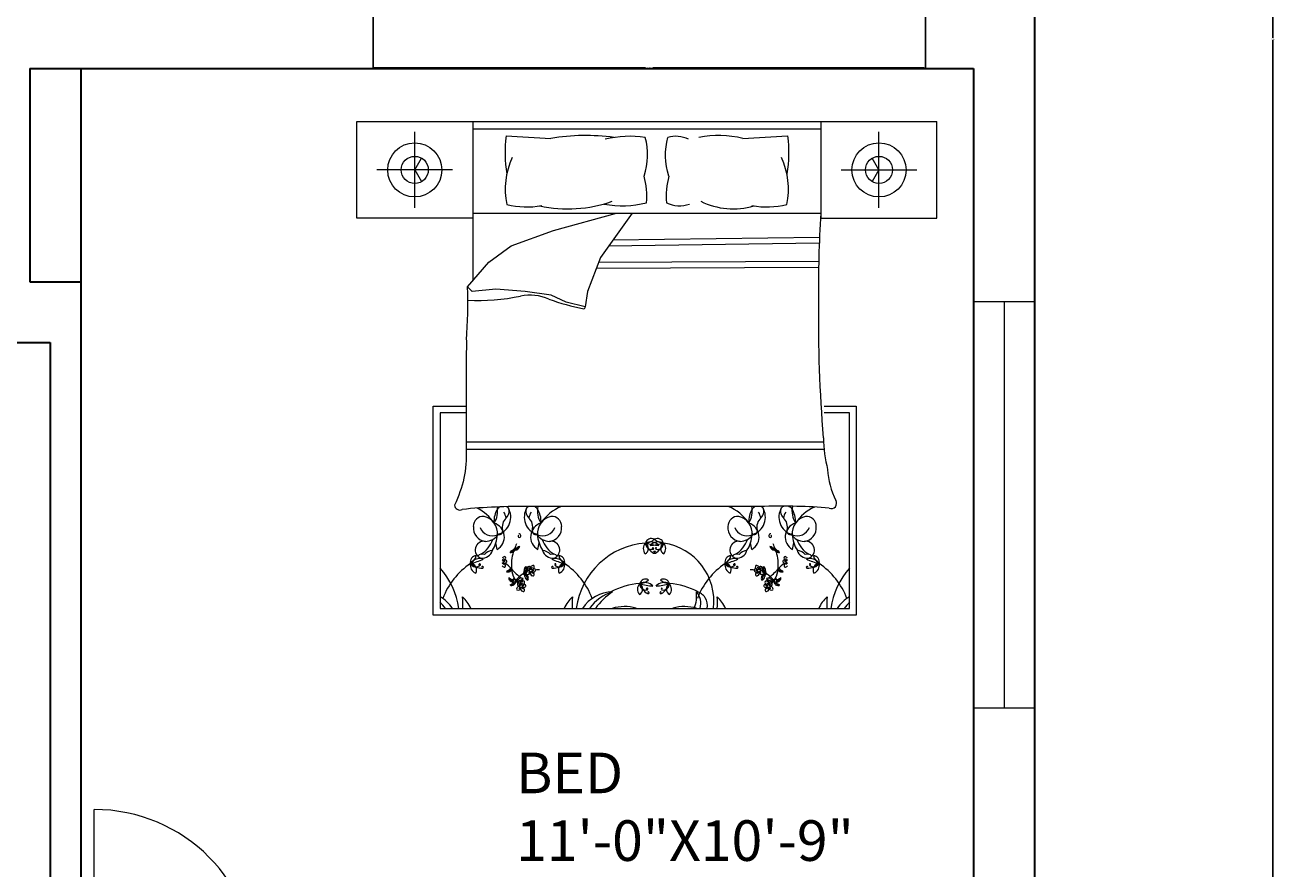
# Model space of a CAD drawing. Units: inches. Extents: x -59 to 444, y -680 to 63.
# Tile 7 of 9: x 260 to 444, y -431 to -306. Entities that reach past the tile are written whole.
import ezdxf

# ---------------------------------------------------------------- set-up
doc = ezdxf.new("R2010")
doc.units = ezdxf.units.IN
doc.header["$MEASUREMENT"] = 0
for name, color, linetype, lineweight in [('A-ANNO-DIMS', 2, 'Continuous', 18), ('A-AREA-IDEN', 7, 'Continuous', 18), ('A-DOOR', 3, 'Continuous', 18), ('A-FLOR-EVTR', 7, 'Continuous', 30), ('A-FURN', 8, 'Continuous', 13), ('A-GLAZ', 4, 'Continuous', 18), ('A-WALL', 7, 'Continuous', 35)]:
    doc.layers.add(name, color=color, linetype=linetype, lineweight=lineweight)
doc.styles.get("Standard").update_dxf_attribs({"font": 'arial.ttf'})
doc.dimstyles.get("Standard").update_dxf_attribs({"dimtxt": 0.18, "dimasz": 0.18, "dimexe": 0.18, "dimexo": 0.0625, "dimgap": 0.09, "dimtad": 0, "dimtih": 1, "dimtoh": 1, "dimdec": 0, "dimzin": 0, "dimdsep": 46, "dimlunit": 3, "dimtxsty": 'Standard', "dimcen": 0.09, "dimadec": 0, "dimazin": 0, "dimtfac": 1, "dimtdec": 0, "dimtofl": 0, "dimtmove": 0, "dimatfit": 3, "dimfxl": 1, "dimtolj": 1, "dimtzin": 0, "dimarcsym": 0})

# ---------------------------------------------------------------- blocks, each defined once
blk = doc.blocks.new('BED-SET-73')
for p, q in [((0, 72.95), (85.77, 72.95)), ((17.15, 72.95), (17.15, 49.4)), ((8.58, 60.19), (8.58, 71.4)), ((68.62, 71.84), (17.15, 71.84)), ((77.2, 60.19), (77.2, 71.4)), ((14.18, 65.8), (2.97, 65.8)), ((71.59, 65.8), (82.8, 65.8)), ((17.15, 59.39), (68.62, 59.39)), ((29.07, 56.84), (38.42, 59.39)), ((40.72, 59.39), (36.02, 52.85)), ((22.81, 54.58), (29.07, 56.84)), ((68.39, 55.83), (37.85, 55.4)), ((19.51, 52.15), (22.81, 54.58)), ((68.36, 54.95), (37.21, 54.51)), ((16.39, 48.51), (19.51, 52.15)), ((36.02, 52.85), (34.11, 47.81)), ((68.31, 52.25), (35.74, 52.12)), ((68.32, 51.37), (35.4, 51.23)), ((17.08, 47.81), (16.39, 48.51)), ((20.56, 48.16), (17.08, 47.81)), ((24.9, 47.81), (20.56, 48.16)), ((28.72, 47.29), (24.9, 47.81)), ((30.98, 46.25), (28.72, 47.29)), ((33.76, 45.56), (30.98, 46.25)), ((34.11, 47.81), (33.76, 45.56)), ((11.32, 30.9), (16.17, 30.9)), ((11.32, 0), (11.32, 30.9)), ((16.17, 29.9), (12.32, 29.9)), ((12.32, 29.9), (12.32, 0.99)), ((72.86, 29.9), (69.08, 29.9)), ((69.1, 30.9), (73.85, 30.9)), ((72.86, 0.99), (72.86, 29.9)), ((73.85, 30.9), (73.85, 0)), ((69.01, 25.55), (16.17, 25.55)), ((69.09, 24.48), (16.17, 24.48)), ((60.3, 16.05), (25.47, 16.05)), ((20.77, 9.69), (20.58, 10.66)), ((26.76, 9.69), (26.95, 10.66)), ((58.41, 9.69), (58.22, 10.66)), ((64.41, 9.69), (64.6, 10.66)), ((73.85, 0), (11.32, 0)), ((12.32, 0.99), (72.86, 0.99))]:
    blk.add_line(p, q)
for points in [[(17.15, 58.65), (0, 58.65), (0, 72.95)], [(68.62, 72.95), (68.62, 58.65), (85.77, 58.65), (85.77, 72.95)], [(8.58, 65.8), (9.58, 67.53)], [(77.2, 65.8), (76.2, 67.53)], [(8.58, 65.8), (9.58, 64.06)], [(77.2, 65.8), (76.2, 64.06)]]:
    blk.add_lwpolyline(points)
for points in [[(22.08, 70.81, 0.074897), (22.19, 65.21, -0.472817)], [(42.49, 64.89, 0.14099), (42.66, 70.61, 0.235245)], [(46.15, 64.89, -0.14099), (45.98, 70.61, -0.235245)], [(63.69, 70.81, -0.074897), (63.59, 65.21, 0.472817)], [(16.21, 40.65, 0.001242), (16.17, 24.38, -0.127202), (14.45, 16.27)], [(68.99, 26.22, 0.056112), (69.61, 21.51, 0.095341), (70.81, 16.96)]]:
    blk.add_lwpolyline(points, format="xyb")
for centre, radius in [((8.58, 65.8), 4), ((77.2, 65.8), 4), ((8.58, 65.8), 2), ((77.2, 65.8), 2), ((25.72, 6.58), 0.218), ((59.45, 6.58), 0.218), ((24.29, 4.28), 0.218), ((60.88, 4.28), 0.218)]:
    blk.add_circle(centre, radius)
for centre, radius, start, end in [((69.36, 887.1), 817.66, 266.68521, 267.14978), ((33.83, 39.77), 31.11, 82.2196, 99.497), ((40.4, 55.49), 15.28, 81.5249, 103.96), ((47.15, 66.53), 4.24, 63.3437, 106.1026), ((53.51, 55.8), 15.08, 76.3427, 101.1841), ((16.41, 887.1), 817.66, 272.85022, 273.31479), ((33.01, 62.96), 11.06, 155.1316, 191.7583), ((52.76, 62.96), 11.06, 348.2417, 24.8684), ((32.37, 62.02), 10.51, 354.0129, 15.8293), ((56.26, 62.02), 10.51, 164.1707, 185.9871), ((31.19, 79.98), 19.94, 258.0397, 289.2615), ((55.67, 70.96), 10.92, 243.8761, 286.1746), ((25.14, 71.81), 11.49, 255.1039, 281.0369), ((39.26, 75.63), 15.13, 259.8617, 283.6238), ((47.73, 65.05), 4.55, 245.0183, 288.5407), ((60.63, 71.81), 11.49, 258.9631, 284.8961), ((222.38, 48.91), 154.12, 176.1, 180.9282), ((-62.26, 46.38), 78.68, 355.8294, 1.553), ((17.85, 78.88), 32.37, 267.4519, 281.3392), ((25.59, 40.3), 6.98, 66.2616, 101.3392), ((39.72, 77.97), 33.26, 250.1194, 259.3383), ((269.3, 43.3), 201.05, 179.1145, 184.8735), ((33.57, 45.49), 0.207, 268.8623, 19.7536), ((70.16, 16.52), 0.782, 246.5219, 33.8264), ((15.24, 16.32), 0.791, 183.98, 297.3412), ((24.45, -73.23), 89.29, 89.3433, 95.6887), ((14.9, 10.01), 6.49, 33.6671, 63.2997), ((23.6, 13.88), 3.31, 145.785, 184.7304), ((17.28, 15.42), 3.55, 328.8218, 9.1554), ((21.68, 15.1), 1.03, 120.0293, 142.325), ((20.04, 14.5), 2.73, 289.2822, 29.1751), ((19.62, 14), 2.47, 7.436, 29.9149), ((21.25, 15.31), 1.28, 311.5653, 23.8354), ((21.68, 15.1), 1.03, 44.4517, 63.558), ((27.5, 14.5), 2.73, 150.8249, 250.7178), ((26.28, 15.31), 1.28, 156.1646, 228.4347), ((25.85, 15.1), 1.03, 113.229, 135.5483), ((27.91, 14), 2.47, 150.0851, 172.564), ((25.85, 15.1), 1.03, 37.675, 66.7144), ((23.93, 13.88), 3.31, 355.2696, 34.215), ((30.25, 15.42), 3.55, 169.7133, 211.1782), ((32.63, 10.01), 6.49, 111.4941, 146.3329), ((52.55, 10.01), 6.49, 33.6671, 68.5059), ((61.25, 13.88), 3.31, 145.785, 184.7304), ((54.93, 15.42), 3.55, 328.8218, 10.2867), ((59.33, 15.1), 1.03, 113.2856, 142.325), ((57.68, 14.5), 2.73, 289.2822, 29.1751), ((57.27, 14), 2.47, 7.436, 29.9149), ((59.33, 15.1), 1.03, 44.4517, 66.7144), ((58.89, 15.31), 1.28, 311.5653, 23.8354), ((62.93, -67.37), 83.47, 85.2402, 91.8035), ((65.14, 14.5), 2.73, 150.8249, 250.7178), ((63.93, 15.31), 1.28, 156.1646, 228.4347), ((63.49, 15.1), 1.03, 106.6343, 135.5483), ((65.55, 14), 2.47, 150.0851, 172.564), ((63.49, 15.1), 1.03, 37.675, 72.5814), ((61.57, 13.88), 3.31, 355.2696, 34.215), ((67.89, 15.42), 3.55, 169.249, 211.1782), ((70.27, 10.01), 6.49, 113.6453, 146.3329), ((19.28, 12.92), 2.05, 174.9449, 262.8857), ((18.68, 13.13), 1.45, 84.4856, 181.0538), ((20.08, 13.7), 1.99, 201.5819, 291.4221), ((18.24, 12.06), 2.58, 355.2933, 76.921), ((19.7, 11.54), 2.13, 299.9085, 73.1337), ((23.27, 13.03), 1.76, 131.5653, 195.1471), ((24.26, 13.03), 1.76, 344.8529, 48.4347), ((27.83, 11.54), 2.13, 106.8663, 240.0915), ((29.29, 12.06), 2.58, 103.079, 184.7067), ((27.45, 13.7), 1.99, 248.5779, 338.4181), ((28.25, 12.92), 2.05, 277.1143, 5.0551), ((28.85, 13.13), 1.45, 358.9462, 95.5144), ((56.92, 12.92), 2.05, 174.9449, 262.8857), ((56.33, 13.13), 1.45, 84.4856, 181.0538), ((57.73, 13.7), 1.99, 201.5819, 291.4221), ((55.88, 12.06), 2.58, 355.2933, 76.921), ((57.35, 11.54), 2.13, 299.9085, 73.1337), ((60.91, 13.03), 1.76, 131.5653, 195.1471), ((61.91, 13.03), 1.76, 344.8529, 48.4347), ((65.47, 11.54), 2.13, 106.8663, 240.0915), ((66.94, 12.06), 2.58, 103.079, 184.7067), ((65.09, 13.7), 1.99, 248.5779, 338.4181), ((65.9, 12.92), 2.05, 277.1143, 5.0551), ((66.49, 13.13), 1.45, 358.9462, 95.5144), ((16.25, 12.45), 4.05, 301.2614, 341.7045), ((18.92, 13.38), 2.49, 272.3591, 324.0401), ((16.22, 12.13), 4.6, 326.2883, 356.5076), ((23.6, 13.88), 3.31, 212.7011, 216.3445), ((21.05, 12.43), 0.532, 257.3041, 15.1471), ((24.01, 11.63), 0.165, 102.7051, 280.4384), ((23.99, 11.73), 0.269, 280.4384, 100.4136), ((26.48, 12.43), 0.532, 164.8529, 282.6959), ((23.93, 13.88), 3.31, 323.6555, 327.2989), ((28.61, 13.38), 2.49, 215.9599, 267.6409), ((31.31, 12.13), 4.6, 183.4924, 213.7117), ((31.28, 12.45), 4.05, 198.2955, 238.7386), ((43.57, 10.39), 0.929, 63.0274, 163.8037), ((42.63, 12.56), 1.91, 271.4585, 315.3727), ((44.46, 10.39), 0.929, 16.1963, 116.9726), ((45.4, 12.56), 1.91, 224.6273, 268.5415), ((53.9, 12.45), 4.05, 301.2614, 341.7045), ((56.57, 13.38), 2.49, 272.3591, 324.0401), ((53.86, 12.13), 4.6, 326.2883, 356.5076), ((61.25, 13.88), 3.31, 212.7011, 216.3445), ((58.7, 12.43), 0.532, 257.3041, 15.1471), ((61.18, 11.73), 0.269, 79.5864, 259.5616), ((61.16, 11.63), 0.165, 259.5616, 77.2949), ((64.12, 12.43), 0.532, 164.8529, 282.6959), ((61.57, 13.88), 3.31, 323.6555, 327.2989), ((66.25, 13.38), 2.49, 215.9599, 267.6409), ((68.96, 12.13), 4.6, 183.4924, 213.7117), ((68.92, 12.45), 4.05, 198.2955, 238.7386), ((18.81, 9.62), 1.29, 80.264, 250.8688), ((18.5, 10.01), 1.61, 265.969, 344.3045), ((20.23, 7.87), 1.71, 96.1662, 141.5825), ((23.06, 9.07), 0.45, 101.3256, 154.4621), ((22.42, 10.6), 1.36, 280.2588, 300.656), ((22.73, 11.68), 2.42, 268.3264, 277.1302), ((29.96, 7.31), 7.1, 163.5842, 183.8277), ((22.12, 10.6), 1.38, 308.2101, 316.3071), ((22.97, 9.69), 0.412, 278.3432, 4.2869), ((22.74, 10.05), 0.719, 300.656, 332.6341), ((23.28, 9.58), 0.175, 55.7657, 157.4417), ((29.96, 7.31), 7.1, 153.0032, 159.8941), ((23.55, 9.74), 0.175, 84.3784, 186.0543), ((23.39, 10.44), 0.719, 269.1859, 301.164), ((23.6, 10.07), 0.412, 237.5332, 323.4768), ((23.2, 11.24), 1.38, 285.5129, 293.6099), ((24.1, 9.69), 0.45, 87.3579, 140.4944), ((23.06, 10.99), 1.36, 301.164, 321.5612), ((21.96, 11.22), 2.42, 324.6898, 333.4936), ((27.3, 7.87), 1.71, 38.4175, 83.8338), ((29.03, 10.01), 1.61, 195.6955, 274.031), ((28.72, 9.62), 1.29, 289.1312, 99.736), ((43.55, -0.52), 11.2, 94.4623, 172.255), ((43.6, 9.82), 1.24, 137.7873, 219.1145), ((42.19, 9.86), 0.935, 298.5391, 58.3627), ((43.41, 9.04), 1.77, 45.5411, 114.3101), ((45.03, 18.13), 7.84, 252.593, 267.2582), ((43.6, 10.62), 0.916, 177.7585, 283.852), ((45.36, 11.57), 2.83, 198.9159, 238.011), ((44.62, 9.04), 1.77, 65.6899, 134.4589), ((43.01, 18.13), 7.84, 272.7418, 287.407), ((43.79, 9.84), 0.121, 283.852, 219.9245), ((43.94, 9.29), 0.139, 238.011, 71.5592), ((43.96, 9.35), 0.0676, 71.5592, 188.0167), ((44.1, 9.29), 0.139, 108.4408, 301.989), ((44.08, 9.35), 0.0676, 351.9833, 108.4408), ((44.23, 9.89), 0.073, 320.1909, 256.0209), ((42.67, 11.57), 2.83, 301.989, 341.0841), ((44.44, 10.62), 0.916, 256.148, 2.2415), ((45.84, 9.86), 0.935, 121.6373, 241.4609), ((44.43, 9.82), 1.24, 320.8855, 42.2127), ((44.12, 2.07), 8.67, 352.8636, 81.8197), ((56.45, 9.62), 1.29, 80.264, 250.8688), ((56.14, 10.01), 1.61, 265.969, 344.3045), ((57.87, 7.87), 1.71, 96.1662, 141.5825), ((62.12, 10.99), 1.36, 218.4388, 238.836), ((61.07, 9.69), 0.45, 39.5056, 92.6421), ((63.22, 11.22), 2.42, 206.5064, 215.3102), ((61.58, 10.07), 0.412, 216.5232, 302.4668), ((61.79, 10.44), 0.719, 238.836, 270.8141), ((61.97, 11.24), 1.38, 246.3901, 254.4871), ((55.22, 7.31), 7.1, 20.1059, 26.9968), ((61.62, 9.74), 0.175, 353.9457, 95.6216), ((61.89, 9.58), 0.175, 22.5583, 124.2343), ((62.21, 9.69), 0.412, 175.7131, 261.6568), ((62.43, 10.05), 0.719, 207.3659, 239.344), ((55.22, 7.31), 7.1, 356.1723, 16.4158), ((63.05, 10.6), 1.38, 223.6929, 231.7899), ((62.76, 10.6), 1.36, 239.344, 259.7412), ((62.45, 11.68), 2.42, 262.8698, 271.6736), ((62.11, 9.07), 0.45, 25.5379, 78.6744), ((66.68, 10.01), 1.61, 195.6955, 274.031), ((64.95, 7.87), 1.71, 38.4175, 83.8338), ((66.37, 9.62), 1.29, 289.1312, 99.736), ((23.14, -1.62), 11.2, 124.3865, 158.5908), ((18.03, 7.36), 1.24, 167.7115, 249.0387), ((17.72, 7.84), 0.929, 92.9516, 193.728), ((15.82, 9.25), 1.91, 301.3827, 345.2969), ((18.25, 6.59), 1.77, 75.4653, 144.2343), ((15.12, 15.27), 7.84, 282.5173, 297.1824), ((16.79, 6.69), 0.935, 328.4633, 88.2869), ((18.68, 9.75), 2.83, 228.8402, 267.9352), ((17.62, 8.05), 0.916, 207.6827, 313.7762), ((18.54, 8.23), 0.789, 63.9755, 143.2681), ((18.17, 7.47), 0.121, 313.7762, 249.7183), ((21.79, 8.22), 0.364, 101.5637, 142.6358), ((21.49, 7.88), 0.218, 273.2768, 86.7232), ((21.74, 8.09), 0.209, 91.1081, 181.8675), ((22.18, 7.96), 0.663, 203.4276, 227.6104), ((21.96, 7.67), 0.452, 80.3487, 133.6538), ((21.88, 8.04), 0.357, 229.7889, 317.6792), ((21.5, 8.5), 0.525, 288.7263, 352.5032), ((21.48, 7.28), 0.508, 355.053, 68.3618), ((21.88, 7.2), 0.715, 83.0852, 105.7171), ((21.86, 8.48), 0.169, 345.2356, 144.9248), ((16.93, 1.27), 8.14, 43.1541, 52.0459), ((22.01, 7.93), 0.188, 317.6792, 80.3487), ((28.99, 8.23), 0.789, 36.7319, 116.0245), ((29.28, 6.59), 1.77, 35.7657, 104.5347), ((32.42, 15.27), 7.84, 242.8176, 257.4827), ((28.85, 9.75), 2.83, 272.0648, 311.1598), ((29.91, 8.05), 0.916, 226.2238, 332.3173), ((29.37, 7.52), 0.073, 290.2667, 226.2271), ((30.74, 6.69), 0.935, 91.7131, 211.5367), ((29.81, 7.84), 0.929, 346.272, 87.0484), ((31.71, 9.25), 1.91, 194.7031, 238.6173), ((29.5, 7.36), 1.24, 290.9613, 12.2885), ((24.39, -1.62), 11.2, 21.4092, 55.6135), ((60.78, -1.62), 11.2, 124.3865, 158.5908), ((55.36, 7.84), 0.929, 92.9516, 193.728), ((55.67, 7.36), 1.24, 167.7115, 249.0387), ((53.46, 9.25), 1.91, 301.3827, 345.2969), ((55.9, 6.59), 1.77, 75.4653, 144.2343), ((52.76, 15.27), 7.84, 282.5173, 297.1824), ((55.27, 8.05), 0.916, 207.6827, 313.7762), ((56.32, 9.75), 2.83, 228.8402, 267.9352), ((54.43, 6.69), 0.935, 328.4633, 88.2869), ((56.19, 8.23), 0.789, 63.9755, 143.2681), ((55.82, 7.47), 0.121, 313.7762, 249.7183), ((68.25, 1.27), 8.14, 127.9541, 136.8459), ((63.17, 7.93), 0.188, 99.6513, 222.3208), ((63.29, 8.04), 0.357, 222.3208, 310.2111), ((63.21, 7.67), 0.452, 46.3462, 99.6513), ((63.32, 8.48), 0.169, 35.0752, 194.7644), ((63.68, 8.5), 0.525, 187.4968, 251.2737), ((63.69, 7.28), 0.508, 111.6382, 184.947), ((63.3, 7.2), 0.715, 74.2829, 96.9148), ((63.43, 8.09), 0.209, 358.1325, 88.8919), ((63, 7.96), 0.663, 312.3896, 336.5724), ((63.38, 8.22), 0.364, 37.3642, 78.4363), ((63.69, 7.88), 0.218, 93.2768, 266.7232), ((66.63, 8.23), 0.789, 36.7319, 116.0245), ((66.93, 6.59), 1.77, 35.7657, 104.5347), ((70.06, 15.27), 7.84, 242.8176, 257.4827), ((66.5, 9.75), 2.83, 272.0648, 311.1598), ((67.55, 8.05), 0.916, 226.2238, 332.3173), ((67.01, 7.52), 0.073, 290.2667, 226.2271), ((68.39, 6.69), 0.935, 91.7131, 211.5367), ((69.36, 9.25), 1.91, 194.7031, 238.6173), ((67.46, 7.84), 0.929, 346.272, 87.0484), ((67.15, 7.36), 1.24, 290.9613, 12.2885), ((62.04, -1.62), 11.2, 21.4092, 55.6135), ((3.98, -0.52), 11.2, 7.745, 41.8856), ((18.57, 7.13), 0.0676, 101.4834, 217.9409), ((18.58, 7.06), 0.139, 267.9352, 101.4834), ((21.79, 7.48), 0.361, 217.7621, 259.0403), ((21.82, 7.25), 0.168, 232.4737, 355.053), ((22.55, 6.19), 0.45, 101.3256, 154.4621), ((21.91, 7.71), 1.36, 280.2588, 300.656), ((22.22, 8.8), 2.42, 268.3264, 277.1302), ((21.61, 7.71), 1.38, 308.2101, 316.3071), ((22.46, 6.81), 0.412, 278.3432, 4.2869), ((22.23, 7.17), 0.719, 300.656, 332.6341), ((22.77, 6.69), 0.175, 55.7657, 157.4417), ((26.42, 7.13), 3.56, 184.756, 209.2041), ((31.54, 14.71), 11.72, 222.2412, 232.1744), ((26.78, 2.4), 4.27, 120.544, 139.818), ((24.58, 6.68), 0.605, 272.8499, 356.1226), ((24.05, 6.91), 0.996, 304.5369, 16.3699), ((24.16, 6.45), 0.586, 321.7607, 7.9252), ((24.28, 5.61), 0.586, 8.7227, 54.8872), ((24.31, 5.14), 0.996, 0.278, 72.111), ((25.43, 6.63), 0.704, 127.3105, 187.9252), ((24.76, 5.5), 0.605, 20.5253, 88.5375), ((25.55, 5.8), 0.704, 188.7227, 249.3375), ((24.47, 6.71), 0.723, 355.0106, 41.658), ((25.26, 6.17), 0.216, 148.0499, 225.6268), ((26.78, 2.4), 4.27, 113.0501, 113.8477), ((25.66, 5.92), 0.689, 104.7558, 148.0499), ((25.28, 6.42), 0.431, 247.4086, 351.4386), ((25.48, 6.89), 0.298, 126.1046, 271.4281), ((25.45, 6.97), 0.214, 353.7526, 131.7054), ((24.65, 5.45), 0.723, 334.9899, 21.6373), ((25.4, 6.4), 0.145, 262.906, 7.132), ((25.25, 6.71), 0.301, 0.0645, 61.1507), ((25.32, 6.97), 0.344, 311.8413, 355.7877), ((26.03, 6.92), 0.364, 101.5637, 176.365), ((26.02, 6.18), 0.361, 151.2196, 259.0403), ((25.98, 6.79), 0.209, 91.1081, 181.8675), ((26.41, 6.66), 0.663, 203.4276, 227.6104), ((26.2, 6.37), 0.452, 80.3487, 133.6538), ((26.12, 6.74), 0.357, 229.7889, 317.6792), ((25.73, 7.21), 0.525, 288.7263, 352.5032), ((25.72, 5.99), 0.508, 355.053, 68.3618), ((26.11, 5.9), 0.715, 83.0852, 105.7171), ((26.09, 7.18), 0.169, 345.2356, 144.9248), ((26.05, 5.96), 0.168, 232.4737, 355.053), ((26.24, 6.63), 0.188, 317.6792, 80.3487), ((26.78, 2.4), 4.27, 87.1071, 94.7585), ((28.95, 7.06), 0.139, 78.5166, 272.0648), ((28.96, 7.13), 0.0676, 322.0591, 78.5166), ((56.21, 7.13), 0.0676, 101.4834, 217.9409), ((56.23, 7.06), 0.139, 267.9352, 101.4834), ((58.39, 2.4), 4.27, 85.2415, 92.8929), ((58.93, 6.63), 0.188, 99.6513, 222.3208), ((59.06, 6.74), 0.357, 222.3208, 310.2111), ((58.98, 6.37), 0.452, 46.3462, 99.6513), ((59.09, 7.18), 0.169, 35.0752, 194.7644), ((59.44, 7.21), 0.525, 187.4968, 251.2737), ((59.46, 5.99), 0.508, 111.6382, 184.947), ((59.12, 5.96), 0.168, 184.947, 307.5263), ((59.06, 5.9), 0.715, 74.2829, 96.9148), ((59.2, 6.79), 0.209, 358.1325, 88.8919), ((58.77, 6.66), 0.663, 312.3896, 336.5724), ((59.15, 6.92), 0.364, 3.635, 78.4363), ((59.15, 6.18), 0.361, 280.9597, 28.7804), ((59.9, 6.42), 0.431, 188.5614, 292.5914), ((59.73, 6.97), 0.214, 48.2946, 186.2474), ((59.86, 6.97), 0.344, 184.2123, 228.1587), ((59.93, 6.71), 0.301, 118.8493, 179.9355), ((59.78, 6.4), 0.145, 172.868, 277.094), ((59.69, 6.89), 0.298, 268.5719, 53.8954), ((59.51, 5.92), 0.689, 31.9501, 75.2442), ((60.53, 5.45), 0.723, 158.3627, 205.0101), ((60.42, 5.5), 0.605, 91.4625, 159.4747), ((60.87, 5.14), 0.996, 107.889, 179.722), ((59.62, 5.8), 0.704, 290.6625, 351.2773), ((60.71, 6.71), 0.723, 138.342, 184.9894), ((60.59, 6.68), 0.605, 183.8774, 267.1501), ((58.39, 2.4), 4.27, 66.1523, 66.9499), ((59.91, 6.17), 0.216, 314.3732, 31.9501), ((61.12, 6.91), 0.996, 163.6301, 235.4631), ((59.74, 6.63), 0.704, 352.0748, 52.6895), ((60.9, 5.61), 0.586, 125.1128, 171.2773), ((61.02, 6.45), 0.586, 172.0748, 218.2393), ((58.39, 2.4), 4.27, 40.182, 59.456), ((53.63, 14.71), 11.72, 307.8256, 317.7588), ((58.76, 7.13), 3.56, 330.7959, 355.244), ((62.41, 6.69), 0.175, 22.5583, 124.2343), ((62.72, 6.81), 0.412, 175.7131, 261.6568), ((62.95, 7.17), 0.719, 207.3659, 239.344), ((63.56, 7.71), 1.38, 223.6929, 231.7899), ((63.27, 7.71), 1.36, 239.344, 259.7412), ((62.96, 8.8), 2.42, 262.8698, 271.6736), ((62.62, 6.19), 0.45, 25.5379, 78.6744), ((63.36, 7.25), 0.168, 184.947, 307.5263), ((63.39, 7.48), 0.361, 280.9597, 322.2379), ((66.59, 7.06), 0.139, 78.5166, 272.0648), ((66.61, 7.13), 0.0676, 322.0591, 78.5166), ((81.2, -0.52), 11.2, 138.1144, 172.255), ((22.71, 5.4), 0.244, 146.8636, 236.9021), ((26.14, 10.77), 6.38, 235.1882, 238.8844), ((23.12, 5.75), 0.66, 199.4799, 267.6828), ((23.05, 5.5), 0.569, 212.8155, 277.3992), ((22.72, 5.12), 0.66, 266.9701, 338.2913), ((19.24, 9.83), 6.38, 302.6784, 306.3746), ((22.89, 4.6), 0.244, 214.3538, 304.3923), ((22.98, 5.52), 0.253, 238.8844, 314.2646), ((22.92, 4.96), 0.569, 280.3057, 17.1958), ((22.87, 4.9), 0.253, 306.3746, 21.7548), ((23.29, 5.06), 0.191, 19.3605, 201.7548), ((23.29, 5.2), 0.191, 311.8703, 134.2646), ((26.87, 3.47), 3.8, 153.7819, 158.2913), ((23.84, 6.07), 0.996, 247.2305, 319.0635), ((23.51, 5.73), 0.586, 264.4544, 310.6188), ((23.94, 5.5), 0.605, 218.3208, 298.8162), ((26.42, 7.13), 3.56, 214.0033, 222.4917), ((23.84, 3.87), 0.216, 148.0499, 225.6268), ((24.24, 3.62), 0.689, 104.7558, 148.0499), ((23.85, 4.11), 0.431, 247.4086, 351.4386), ((24.05, 4.58), 0.298, 126.1046, 271.4281), ((24.02, 4.66), 0.214, 353.7526, 131.7054), ((24.35, 4.75), 0.704, 70.0041, 130.6188), ((23.97, 4.1), 0.145, 262.906, 7.132), ((23.82, 4.41), 0.301, 0.0645, 61.1507), ((23.89, 4.67), 0.344, 311.8413, 355.7877), ((23.89, 5.61), 0.723, 297.7043, 344.3516), ((24.6, 4.62), 0.364, 101.5637, 176.365), ((24.59, 3.88), 0.361, 151.2196, 259.0403), ((24.55, 4.49), 0.209, 91.1081, 181.8675), ((24.98, 4.36), 0.663, 203.4276, 227.6104), ((24.77, 4.07), 0.452, 80.3487, 133.6538), ((24.69, 4.44), 0.357, 229.7889, 317.6792), ((24.3, 4.9), 0.525, 288.7263, 352.5032), ((24.29, 3.68), 0.508, 355.053, 68.3618), ((24.68, 3.6), 0.715, 83.0852, 105.7171), ((24.66, 4.88), 0.169, 345.2356, 144.9248), ((24.81, 4.33), 0.188, 317.6792, 80.3487), ((42.7, -6.51), 11.2, 94.4623, 117.4146), ((42.74, 3.82), 1.24, 137.7873, 219.1145), ((41.33, 3.86), 0.935, 298.5391, 58.3627), ((42.72, 4.39), 0.929, 63.0274, 163.8037), ((41.78, 6.56), 1.91, 271.4585, 315.3727), ((42.55, 3.04), 1.77, 45.5411, 114.3101), ((44.5, 5.57), 2.83, 198.9159, 238.011), ((44.17, 12.13), 7.84, 252.593, 267.2582), ((42.74, 4.62), 0.916, 177.7585, 283.852), ((42.93, 3.84), 0.121, 283.852, 219.9245), ((45.48, 3.04), 1.77, 65.6899, 134.4589), ((43.87, 12.13), 7.84, 272.7418, 287.407), ((45.32, 4.39), 0.929, 16.1963, 116.9726), ((46.26, 6.56), 1.91, 224.6273, 268.5415), ((45.09, 3.89), 0.073, 320.1909, 256.0209), ((43.53, 5.57), 2.83, 301.989, 341.0841), ((45.29, 4.62), 0.916, 256.148, 2.2415), ((46.7, 3.86), 0.935, 121.6373, 241.4609), ((45.29, 3.82), 1.24, 320.8855, 42.2127), ((45.34, -6.51), 11.2, 62.5854, 85.5377), ((60.36, 4.33), 0.188, 99.6513, 222.3208), ((60.49, 4.44), 0.357, 222.3208, 310.2111), ((60.4, 4.07), 0.452, 46.3462, 99.6513), ((60.51, 4.88), 0.169, 35.0752, 194.7644), ((60.87, 4.9), 0.525, 187.4968, 251.2737), ((60.89, 3.68), 0.508, 111.6382, 184.947), ((60.49, 3.6), 0.715, 74.2829, 96.9148), ((60.82, 4.75), 0.704, 49.3812, 109.9959), ((61.34, 6.07), 0.996, 220.9365, 292.7695), ((61.28, 5.61), 0.723, 195.6484, 242.2957), ((60.63, 4.49), 0.209, 358.1325, 88.8919), ((60.19, 4.36), 0.663, 312.3896, 336.5724), ((60.58, 4.62), 0.364, 3.635, 78.4363), ((60.58, 3.88), 0.361, 280.9597, 28.7804), ((61.33, 4.11), 0.431, 188.5614, 292.5914), ((61.24, 5.5), 0.605, 241.1838, 321.6792), ((61.16, 4.66), 0.214, 48.2946, 186.2474), ((61.29, 4.67), 0.344, 184.2123, 228.1587), ((61.36, 4.41), 0.301, 118.8493, 179.9355), ((61.2, 4.1), 0.145, 172.868, 277.094), ((61.12, 4.58), 0.298, 268.5719, 53.8954), ((60.94, 3.62), 0.689, 31.9501, 75.2442), ((61.66, 5.73), 0.586, 229.3812, 275.5456), ((58.76, 7.13), 3.56, 317.5083, 325.9967), ((61.34, 3.87), 0.216, 314.3732, 31.9501), ((62.25, 4.96), 0.569, 162.8042, 259.6943), ((61.89, 5.2), 0.191, 45.7354, 228.1297), ((61.89, 5.06), 0.191, 338.2452, 160.6395), ((58.31, 3.47), 3.8, 21.7087, 26.2181), ((62.46, 5.12), 0.66, 201.7087, 273.0299), ((62.2, 5.52), 0.253, 225.7354, 301.1156), ((62.13, 5.5), 0.569, 262.6008, 327.1845), ((62.3, 4.9), 0.253, 158.2452, 233.6254), ((62.05, 5.75), 0.66, 272.3172, 340.5201), ((65.94, 9.83), 6.38, 233.6254, 237.3216), ((62.29, 4.6), 0.244, 235.6077, 325.6462), ((59.03, 10.77), 6.38, 301.1156, 304.8118), ((62.47, 5.4), 0.244, 303.0979, 33.1364), ((9.6, -2.02), 5.46, 33.4617, 60.1116), ((7.63, -3.03), 6.8, 36.3036, 46.4814), ((12.65, -0.75), 4.55, 22.5547, 48.9546), ((0.18, 1.69), 15.5, 357.4081, 3.6519), ((24.63, 3.65), 0.168, 232.4737, 355.053), ((34.88, -0.75), 4.55, 131.0454, 157.4453), ((47.35, 1.69), 15.5, 176.3481, 182.5919), ((37.93, -2.02), 5.46, 91.272, 146.5383), ((39.9, -3.03), 6.8, 107.8504, 143.6964), ((43.47, -4.95), 10.12, 124.0123, 144.053), ((43.08, 3.29), 0.139, 238.011, 71.5592), ((43.1, 3.35), 0.0676, 71.5592, 188.0167), ((44.96, 3.29), 0.139, 108.4408, 301.989), ((44.93, 3.35), 0.0676, 351.9833, 108.4408), ((45.24, 2.86), 5.01, 338.117, 6.6195), ((49.84, 1.47), 2.01, 346.3898, 79.0739), ((48.33, 1.74), 2.54, 342.8609, 41.9049), ((37.82, 1.69), 15.5, 357.4081, 3.6519), ((50.3, -0.75), 4.55, 22.5547, 48.9546), ((60.55, 3.65), 0.168, 184.947, 307.5263), ((72.52, -0.75), 4.55, 131.0454, 157.4453), ((85, 1.69), 15.5, 176.3481, 182.5919), ((75.58, -2.02), 5.46, 119.8884, 146.5383), ((77.54, -3.03), 6.8, 133.5186, 143.6964), ((39.56, -4.9), 6.16, 73.5431, 107.0202), ((42, -8.07), 9.11, 94.3787, 95.6357), ((46.8, -14.31), 16.28, 109.7217, 109.9028), ((48.47, -4.9), 6.16, 72.9798, 106.4569), ((46.03, -8.07), 9.11, 84.3643, 85.6213), ((41.23, -14.31), 16.28, 70.0972, 70.2783)]:
    blk.add_arc(centre, radius, start, end)
blk = doc.blocks.new('WIN-60-W9')
for p, q in [((60, 9), (0, 9)), ((0, 9), (0, 0)), ((60, 0), (60, 9)), ((0, 4.5), (60, 4.5)), ((0, 0), (60, 0))]:
    blk.add_line(p, q)
blk = doc.blocks.new('DOOR-SWING-24')
blk.add_line((24, 0), (0, 0))
blk.add_arc((24, 0), 24, 90, 180)
blk = doc.blocks.new('*D39')
at = {"layer": 'A-ANNO-DIMS', "color": 0, "lineweight": -2, "transparency": 16777216}
for p, q in [((310.95, -298.49), (310.95, -313.01)), ((392.61, -298.49), (392.61, -313.01)), ((311.13, -312.83), (351.25, -312.83)), ((392.43, -312.83), (352.31, -312.83))]:
    blk.add_line(p, q, dxfattribs=at)
at = {"layer": 'A-ANNO-DIMS', "color": 0, "transparency": 16777216}
for points in [[(311.13, -312.8), (311.13, -312.86), (310.95, -312.83)], [(392.43, -312.8), (392.43, -312.86), (392.61, -312.83)]]:
    blk.add_solid(points, dxfattribs=at)
at = {"layer": 'Defpoints', "color": 0, "transparency": 16777216}
for p in [(310.95, -298.42), (392.61, -298.42), (392.61, -312.83)]:
    blk.add_point(p, dxfattribs=at)
at = {"layer": 'A-ANNO-DIMS', "color": 0, "transparency": 16777216, "insert": (351.78, -312.83), "char_height": 0.18, "attachment_point": 5}
blk.add_mtext('\\A1;82 TYP.', dxfattribs=at)
blk = doc.blocks.new('*D47')
at = {"layer": 'A-ANNO-DIMS', "color": 0, "lineweight": -2, "transparency": 16777216}
for p, q in [((267.79, 27.31), (444.16, 27.31)), ((443.98, 27.13), (443.98, -308.38)), ((443.98, -644.26), (443.98, -308.74)), ((267.79, -644.44), (444.16, -644.44))]:
    blk.add_line(p, q, dxfattribs=at)
at = {"layer": 'A-ANNO-DIMS', "color": 0, "transparency": 16777216}
for points in [[(443.95, 27.13), (444.01, 27.13), (443.98, 27.31)], [(443.95, -644.26), (444.01, -644.26), (443.98, -644.44)]]:
    blk.add_solid(points, dxfattribs=at)
at = {"layer": 'Defpoints', "color": 0, "transparency": 16777216}
for p in [(267.73, 27.31), (443.98, 27.31), (267.73, -644.44)]:
    blk.add_point(p, dxfattribs=at)
at = {"layer": 'A-ANNO-DIMS', "color": 0, "transparency": 16777216, "insert": (443.98, -308.56), "char_height": 0.18, "attachment_point": 5}
blk.add_mtext('\\A1;671.8', dxfattribs=at)

msp = doc.modelspace()

# ---------------------------------------------------------------- linework, layer by layer
at = {"layer": 'A-FLOR-EVTR'}
for p, q in [((260.23, -312.94), (260.23, -344.44)), ((260.23, -344.44), (267.73, -344.44))]:
    msp.add_line(p, q, dxfattribs=at)
at = {"layer": 'A-WALL'}
for p, q in [((408.73, 15.56), (408.73, -632.44)), ((260.23, -312.94), (399.73, -312.94)), ((267.73, -312.94), (267.73, -446.44)), ((399.73, -312.94), (399.73, -441.94)), ((159.23, -353.44), (263.23, -353.44)), ((263.23, -353.44), (263.23, -446.44))]:
    msp.add_line(p, q, dxfattribs=at)

# ---------------------------------------------------------------- block references
at = {"layer": 'A-DOOR', "rotation": 270.0000000000001}
msp.add_blockref('DOOR-SWING-24', (269.73, -422.44), dxfattribs=at)
at = {"layer": 'A-FURN'}
msp.add_blockref('BED-SET-73', (308.54, -393.71), dxfattribs=at)
at = {"layer": 'A-GLAZ', "rotation": 269.9999999999999}
msp.add_blockref('WIN-60-W9', (399.73, -347.43), dxfattribs=at)

# ---------------------------------------------------------------- texts
at = {"layer": 'A-AREA-IDEN', "insert": (332.09, -414.04), "char_height": 6, "attachment_point": 1}
msp.add_mtext('BED\\P11\'-0"X10\'-9"', dxfattribs=at)

# ---------------------------------------------------------------- dimensions: what is measured, and where the dimension line sits
at = {"layer": 'A-ANNO-DIMS'}
dim = msp.add_linear_dim(base=(443.9798, 27.314705), p1=(267.7298, -644.435295), p2=(267.7298, 27.314705), angle=90, dimstyle='Standard', override={"dimdec": 1, "dimlfac": 1, "dimrnd": 0, "dimzin": 0, "dimdsep": 46, "dimlunit": 2}, dxfattribs=at)
dim.commit()
dim.dimension.update_dxf_attribs({"geometry": '*D47', "text_midpoint": (443.9798, -308.560295)})
dim = msp.add_linear_dim(base=(392.61, -312.83), p1=(310.95, -298.42), p2=(392.61, -298.42), text='<> TYP.', dimstyle='Standard', override={"dimdec": 0, "dimlfac": 1, "dimrnd": 0, "dimzin": 0, "dimdsep": 46, "dimlunit": 2}, dxfattribs=at)
dim.commit()
dim.dimension.update_dxf_attribs({"geometry": '*D39', "text_midpoint": (351.78, -312.83)})

doc.saveas('drawing.dxf')
